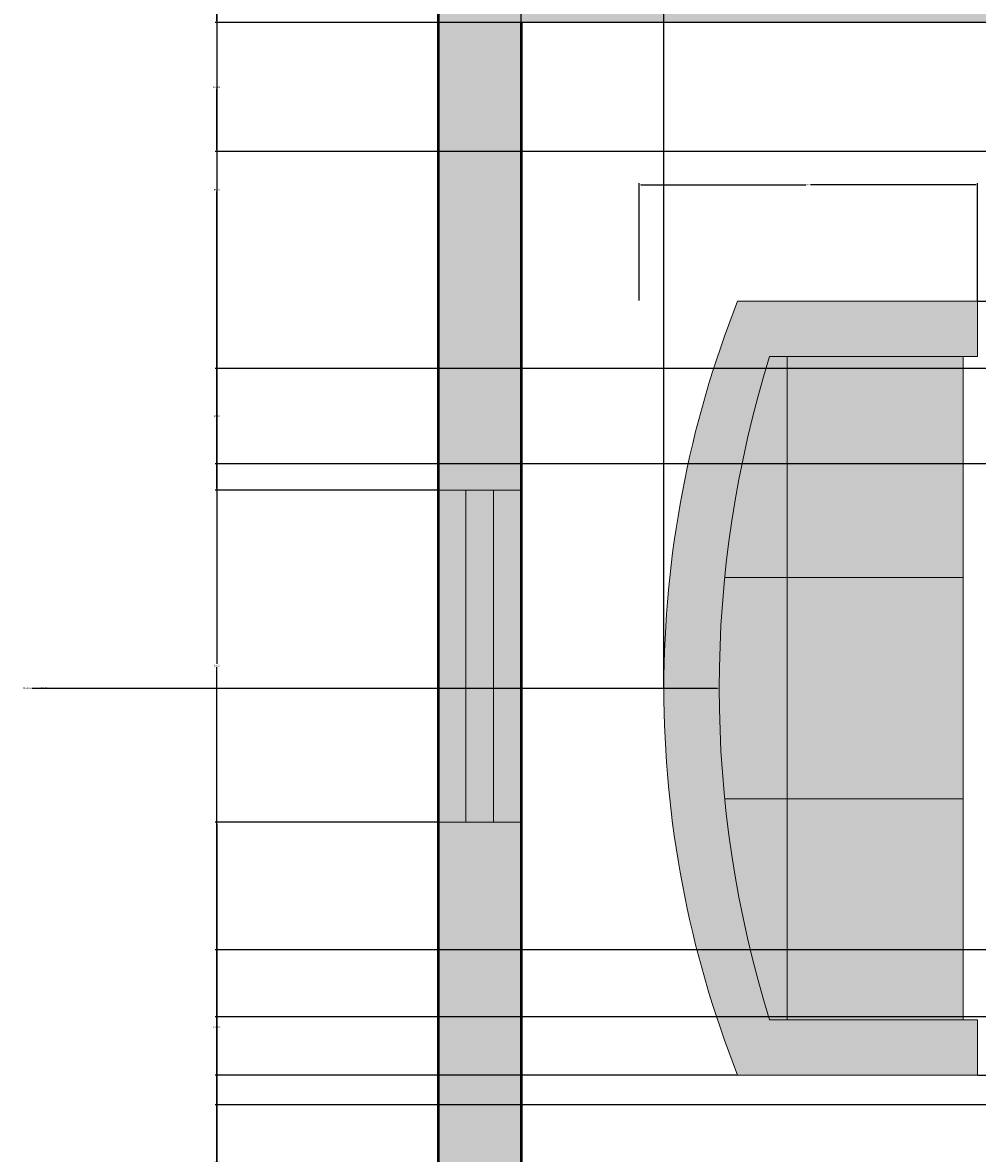
# Model space of a CAD drawing. Units: inches. Extents: x 1201 to 1754, y 247 to 775.
# Tile 2 of 10: x 1201 to 1305, y 435 to 557. Entities that reach past the tile are written whole.
import ezdxf

# ---------------------------------------------------------------- set-up
doc = ezdxf.new("R2010")
doc.units = ezdxf.units.IN
for name, color, linetype, lineweight in [('A-ANNO-DIMS', 2, 'Continuous', 18), ('A-FURN', 8, 'Continuous', 18), ('A-FURN-PATT', 9, 'Continuous', 13), ('A-GLAZ', 4, 'Continuous', 18), ('A-GLAZ-PATT', 9, 'Continuous', 13), ('A-WALL', 7, 'Continuous', 50), ('A-WALL-PATT', 9, 'Continuous', 13)]:
    doc.layers.add(name, color=color, linetype=linetype, lineweight=lineweight)
doc.styles.get("Standard").update_dxf_attribs({"font": 'arial.ttf'})
doc.dimstyles.get("Standard").update_dxf_attribs({"dimtxt": 0.18, "dimasz": 0.18, "dimexe": 0.18, "dimexo": 0.0625, "dimgap": 0.09, "dimtad": 0, "dimtih": 1, "dimtoh": 1, "dimdec": 4, "dimzin": 0, "dimdsep": 46, "dimtxsty": 'Standard', "dimcen": 0.09, "dimadec": 0, "dimazin": 0, "dimtfac": 1, "dimtdec": 4, "dimtofl": 0, "dimtmove": 0, "dimatfit": 3, "dimfxl": 1, "dimtolj": 1, "dimtzin": 0, "dimarcsym": 0})

# ---------------------------------------------------------------- blocks, each defined once
blk = doc.blocks.new('Sofa - Roundback 7 ft.')
for p, q in [((-12.00002, -32.4421), (-12.00003, -6.5971)), ((11.99997, -32.4421), (11.99998, -6.5971)), ((-36.000027, -34), (-36.000027, -11.4696)), ((35.99998, -34), (35.99998, -11.4696)), ((-35.999844, -13.3819), (35.9998, -13.3819)), ((-36.000027, -32.4421), (35.99998, -32.4421))]:
    blk.add_line(p, q)
for points in [[(-36.000027, -34), (-42.000027, -34), (-42.000027, -8)], [(41.99998, -8), (41.99998, -34), (35.99998, -34)]]:
    blk.add_lwpolyline(points)
for centre, radius, start, end in [((0, -114.25), 114.25, 68.43141, 111.5686), ((-0.00001, -127.1968), 121.1968, 72.72033, 107.2797)]:
    blk.add_arc(centre, radius, start, end)
blk = doc.blocks.new('WIN-36IN-PLAN')
for p, q in [((9, 36), (0, 36)), ((3, 0), (3, 36)), ((6, 0), (6, 36))]:
    blk.add_line(p, q)
blk.add_lwpolyline([(0, 36), (0, 0), (9, 0), (9, 36)])
blk = doc.blocks.new('*D37')
at = {"layer": 'A-ANNO-DIMS', "color": 0, "lineweight": -2, "transparency": 16777216}
for p, q in [((1305.08, 527.23), (1317.8, 527.23)), ((1317.62, 527.05), (1317.62, 485.41)), ((1317.62, 443.41), (1317.62, 485.04)), ((1305.08, 443.23), (1317.8, 443.23))]:
    blk.add_line(p, q, dxfattribs=at)
at = {"layer": 'A-ANNO-DIMS', "color": 0, "transparency": 16777216}
for points in [[(1317.59, 527.05), (1317.65, 527.05), (1317.62, 527.23)], [(1317.59, 443.41), (1317.65, 443.41), (1317.62, 443.23)]]:
    blk.add_solid(points, dxfattribs=at)
at = {"layer": 'Defpoints', "color": 0, "transparency": 16777216}
for p in [(1305.02, 527.23), (1317.62, 527.23), (1305.02, 443.23)]:
    blk.add_point(p, dxfattribs=at)
at = {"layer": 'A-ANNO-DIMS', "color": 0, "transparency": 16777216, "insert": (1317.62, 485.23), "char_height": 0.18, "attachment_point": 5}
blk.add_mtext('\\A1;SOFA 84', dxfattribs=at)
blk = doc.blocks.new('*D38')
at = {"layer": 'A-ANNO-DIMS', "color": 0, "lineweight": -2, "transparency": 16777216}
for p, q in [((1268.35, 527.29), (1268.35, 540.01)), ((1305.02, 527.29), (1305.02, 540.01)), ((1268.53, 539.83), (1286.46, 539.83)), ((1304.84, 539.83), (1286.9, 539.83))]:
    blk.add_line(p, q, dxfattribs=at)
at = {"layer": 'A-ANNO-DIMS', "color": 0, "transparency": 16777216}
for points in [[(1268.53, 539.86), (1268.53, 539.8), (1268.35, 539.83)], [(1304.84, 539.86), (1304.84, 539.8), (1305.02, 539.83)]]:
    blk.add_solid(points, dxfattribs=at)
at = {"layer": 'Defpoints', "color": 0, "transparency": 16777216}
for p in [(1268.35, 539.83), (1268.35, 527.23), (1305.02, 527.23)]:
    blk.add_point(p, dxfattribs=at)
at = {"layer": 'A-ANNO-DIMS', "color": 0, "transparency": 16777216, "insert": (1286.68, 539.83), "char_height": 0.18, "attachment_point": 5}
blk.add_mtext('\\A1;37', dxfattribs=at)
blk = doc.blocks.new('*D50')
at = {"layer": 'A-ANNO-DIMS', "color": 0, "lineweight": -2, "transparency": 16777216}
for p, q in [((1255.46, 557.44), (1222.33, 557.44)), ((1222.51, 557.26), (1222.51, 487.87)), ((1222.51, 418.12), (1222.51, 487.51)), ((1255.46, 417.94), (1222.33, 417.94))]:
    blk.add_line(p, q, dxfattribs=at)
at = {"layer": 'A-ANNO-DIMS', "color": 0, "transparency": 16777216}
for points in [[(1222.48, 557.26), (1222.54, 557.26), (1222.51, 557.44)], [(1222.48, 418.12), (1222.54, 418.12), (1222.51, 417.94)]]:
    blk.add_solid(points, dxfattribs=at)
at = {"layer": 'Defpoints', "color": 0, "transparency": 16777216}
for p in [(1255.52, 557.44), (1222.51, 417.94), (1255.52, 417.94)]:
    blk.add_point(p, dxfattribs=at)
at = {"layer": 'A-ANNO-DIMS', "color": 0, "transparency": 16777216, "insert": (1222.51, 487.69), "char_height": 0.18, "attachment_point": 5}
blk.add_mtext('\\A1;139.5', dxfattribs=at)
blk = doc.blocks.new('*D59')
at = {"layer": 'A-ANNO-DIMS', "color": 0, "lineweight": -2, "transparency": 16777216}
for p, q in [((1255.52, 418), (1255.52, 775.14)), ((1255.7, 774.96), (1330.24, 774.96)), ((1405.34, 774.96), (1330.8, 774.96)), ((1405.52, 418), (1405.52, 775.14))]:
    blk.add_line(p, q, dxfattribs=at)
at = {"layer": 'A-ANNO-DIMS', "color": 0, "transparency": 16777216}
for points in [[(1255.7, 774.99), (1255.7, 774.93), (1255.52, 774.96)], [(1405.34, 774.99), (1405.34, 774.93), (1405.52, 774.96)]]:
    blk.add_solid(points, dxfattribs=at)
at = {"layer": 'Defpoints', "color": 0, "transparency": 16777216}
for p in [(1405.52, 774.96), (1255.52, 417.94), (1405.52, 417.94)]:
    blk.add_point(p, dxfattribs=at)
at = {"layer": 'A-ANNO-DIMS', "color": 0, "transparency": 16777216, "insert": (1330.52, 774.96), "char_height": 0.18, "attachment_point": 5}
blk.add_mtext('\\A1;150', dxfattribs=at)
blk = doc.blocks.new('*D70')
at = {"layer": 'A-ANNO-DIMS', "color": 0, "lineweight": -2, "transparency": 16777216}
for p, q in [((1246.46, 470.7), (1222.33, 470.7)), ((1222.51, 470.52), (1222.51, 409.4)), ((1222.51, 347.93), (1222.51, 409.04)), ((1246.46, 347.75), (1222.33, 347.75))]:
    blk.add_line(p, q, dxfattribs=at)
at = {"layer": 'A-ANNO-DIMS', "color": 0, "transparency": 16777216}
for points in [[(1222.48, 470.52), (1222.54, 470.52), (1222.51, 470.7)], [(1222.48, 347.93), (1222.54, 347.93), (1222.51, 347.75)]]:
    blk.add_solid(points, dxfattribs=at)
at = {"layer": 'Defpoints', "color": 0, "transparency": 16777216}
for p in [(1222.51, 470.7), (1246.52, 470.7), (1246.52, 347.75)]:
    blk.add_point(p, dxfattribs=at)
at = {"layer": 'A-ANNO-DIMS', "color": 0, "transparency": 16777216, "insert": (1222.51, 409.22), "char_height": 0.18, "attachment_point": 5}
blk.add_mtext('\\A1;122.95', dxfattribs=at)
blk = doc.blocks.new('*D71')
at = {"layer": 'A-ANNO-DIMS', "color": 0, "lineweight": -2, "transparency": 16777216}
for p, q in [((1246.46, 571.89), (1222.33, 571.89)), ((1222.51, 571.71), (1222.51, 539.47)), ((1222.51, 506.88), (1222.51, 539.11)), ((1246.46, 506.7), (1222.33, 506.7))]:
    blk.add_line(p, q, dxfattribs=at)
at = {"layer": 'A-ANNO-DIMS', "color": 0, "transparency": 16777216}
for points in [[(1222.48, 571.71), (1222.54, 571.71), (1222.51, 571.89)], [(1222.48, 506.88), (1222.54, 506.88), (1222.51, 506.7)]]:
    blk.add_solid(points, dxfattribs=at)
at = {"layer": 'Defpoints', "color": 0, "transparency": 16777216}
for p in [(1222.51, 571.89), (1246.52, 571.89), (1246.52, 506.7)]:
    blk.add_point(p, dxfattribs=at)
at = {"layer": 'A-ANNO-DIMS', "color": 0, "transparency": 16777216, "insert": (1222.51, 539.29), "char_height": 0.18, "attachment_point": 5}
blk.add_mtext('\\A1;65.19', dxfattribs=at)
blk = doc.blocks.new('*D75')
at = {"layer": 'A-ANNO-DIMS', "color": 0, "lineweight": -2, "transparency": 16777216}
for p, q in [((1717.46, 557.44), (1222.33, 557.44)), ((1222.51, 557.26), (1222.51, 550.62)), ((1222.51, 543.62), (1222.51, 550.26)), ((1717.46, 543.44), (1222.33, 543.44))]:
    blk.add_line(p, q, dxfattribs=at)
at = {"layer": 'A-ANNO-DIMS', "color": 0, "transparency": 16777216}
for points in [[(1222.48, 557.26), (1222.54, 557.26), (1222.51, 557.44)], [(1222.48, 543.62), (1222.54, 543.62), (1222.51, 543.44)]]:
    blk.add_solid(points, dxfattribs=at)
at = {"layer": 'Defpoints', "color": 0, "transparency": 16777216}
for p in [(1222.51, 557.44), (1717.52, 557.44), (1717.52, 543.44)]:
    blk.add_point(p, dxfattribs=at)
at = {"layer": 'A-ANNO-DIMS', "color": 0, "transparency": 16777216, "insert": (1222.51, 550.44), "char_height": 0.18, "attachment_point": 5}
blk.add_mtext('\\A1;14.005', dxfattribs=at)
blk = doc.blocks.new('*D83')
at = {"layer": 'A-ANNO-DIMS', "color": 0, "lineweight": -2, "transparency": 16777216}
for p, q in [((1471.46, 561.97), (1222.33, 561.97)), ((1222.51, 561.79), (1222.51, 559.89)), ((1222.51, 557.62), (1222.51, 559.52)), ((1471.46, 557.44), (1222.33, 557.44))]:
    blk.add_line(p, q, dxfattribs=at)
at = {"layer": 'A-ANNO-DIMS', "color": 0, "transparency": 16777216}
for points in [[(1222.48, 561.79), (1222.54, 561.79), (1222.51, 561.97)], [(1222.48, 557.62), (1222.54, 557.62), (1222.51, 557.44)]]:
    blk.add_solid(points, dxfattribs=at)
at = {"layer": 'Defpoints', "color": 0, "transparency": 16777216}
for p in [(1222.51, 561.97), (1471.52, 561.97), (1471.52, 557.44)]:
    blk.add_point(p, dxfattribs=at)
at = {"layer": 'A-ANNO-DIMS', "color": 0, "transparency": 16777216, "insert": (1222.51, 559.71), "char_height": 0.18, "attachment_point": 5}
blk.add_mtext('\\A1;4.528', dxfattribs=at)
blk = doc.blocks.new('*D93')
at = {"layer": 'A-ANNO-DIMS', "color": 0, "lineweight": -2, "transparency": 16777216}
for p, q in [((1278.95, 443.23), (1222.33, 443.23)), ((1222.51, 443.05), (1222.51, 430.77)), ((1222.51, 418.12), (1222.51, 430.4)), ((1255.46, 417.94), (1222.33, 417.94))]:
    blk.add_line(p, q, dxfattribs=at)
at = {"layer": 'A-ANNO-DIMS', "color": 0, "transparency": 16777216}
for points in [[(1222.48, 443.05), (1222.54, 443.05), (1222.51, 443.23)], [(1222.48, 418.12), (1222.54, 418.12), (1222.51, 417.94)]]:
    blk.add_solid(points, dxfattribs=at)
at = {"layer": 'Defpoints', "color": 0, "transparency": 16777216}
for p in [(1222.51, 443.23), (1279.02, 443.23), (1255.52, 417.94)]:
    blk.add_point(p, dxfattribs=at)
at = {"layer": 'A-ANNO-DIMS', "color": 0, "transparency": 16777216, "insert": (1222.51, 430.58), "char_height": 0.18, "attachment_point": 5}
blk.add_mtext('\\A1;25.285', dxfattribs=at)
blk = doc.blocks.new('*D95')
at = {"layer": 'A-ANNO-DIMS', "color": 0, "lineweight": -2, "transparency": 16777216}
for p, q in [((1366.15, 449.58), (1222.33, 449.58)), ((1222.51, 449.4), (1222.51, 433.94)), ((1222.51, 418.12), (1222.51, 433.58)), ((1405.46, 417.94), (1222.33, 417.94))]:
    blk.add_line(p, q, dxfattribs=at)
at = {"layer": 'A-ANNO-DIMS', "color": 0, "transparency": 16777216}
for points in [[(1222.48, 449.4), (1222.54, 449.4), (1222.51, 449.58)], [(1222.48, 418.12), (1222.54, 418.12), (1222.51, 417.94)]]:
    blk.add_solid(points, dxfattribs=at)
at = {"layer": 'Defpoints', "color": 0, "transparency": 16777216}
for p in [(1366.21, 449.58), (1222.51, 417.94), (1405.52, 417.94)]:
    blk.add_point(p, dxfattribs=at)
at = {"layer": 'A-ANNO-DIMS', "color": 0, "transparency": 16777216, "insert": (1222.51, 433.76), "char_height": 0.18, "attachment_point": 5}
blk.add_mtext('\\A1;31.64', dxfattribs=at)
blk = doc.blocks.new('*D96')
at = {"layer": 'A-ANNO-DIMS', "color": 0, "lineweight": -2, "transparency": 16777216}
for p, q in [((1714.98, 456.83), (1222.33, 456.83)), ((1222.51, 456.65), (1222.51, 448.61)), ((1222.51, 440.21), (1222.51, 448.25)), ((1717.46, 440.03), (1222.33, 440.03))]:
    blk.add_line(p, q, dxfattribs=at)
at = {"layer": 'A-ANNO-DIMS', "color": 0, "transparency": 16777216}
for points in [[(1222.48, 456.65), (1222.54, 456.65), (1222.51, 456.83)], [(1222.48, 440.21), (1222.54, 440.21), (1222.51, 440.03)]]:
    blk.add_solid(points, dxfattribs=at)
at = {"layer": 'Defpoints', "color": 0, "transparency": 16777216}
for p in [(1222.51, 456.83), (1715.05, 456.83), (1717.52, 440.03)]:
    blk.add_point(p, dxfattribs=at)
at = {"layer": 'A-ANNO-DIMS', "color": 0, "transparency": 16777216, "insert": (1222.51, 448.43), "char_height": 0.18, "attachment_point": 5}
blk.add_mtext('\\A1;16.793', dxfattribs=at)
blk = doc.blocks.new('*D97')
at = {"layer": 'A-ANNO-DIMS', "color": 0, "lineweight": -2, "transparency": 16777216}
for p, q in [((1255.52, 506.76), (1255.52, 775.14)), ((1255.7, 774.96), (1262.81, 774.96)), ((1270.84, 774.96), (1263.72, 774.96)), ((1271.02, 485.29), (1271.02, 775.14))]:
    blk.add_line(p, q, dxfattribs=at)
at = {"layer": 'A-ANNO-DIMS', "color": 0, "transparency": 16777216}
for points in [[(1255.7, 774.99), (1255.7, 774.93), (1255.52, 774.96)], [(1270.84, 774.99), (1270.84, 774.93), (1271.02, 774.96)]]:
    blk.add_solid(points, dxfattribs=at)
at = {"layer": 'Defpoints', "color": 0, "transparency": 16777216}
for p in [(1271.02, 774.96), (1255.52, 506.7), (1271.02, 485.23)]:
    blk.add_point(p, dxfattribs=at)
at = {"layer": 'A-ANNO-DIMS', "color": 0, "transparency": 16777216, "insert": (1263.27, 774.96), "char_height": 0.18, "attachment_point": 5}
blk.add_mtext('\\A1;15.496', dxfattribs=at)
blk = doc.blocks.new('*D99')
at = {"layer": 'A-ANNO-DIMS', "color": 0, "lineweight": -2, "transparency": 16777216}
for p, q in [((1379.64, 519.9), (1222.33, 519.9)), ((1222.51, 519.72), (1222.51, 514.93)), ((1222.51, 509.76), (1222.51, 514.56)), ((1366.15, 509.58), (1222.33, 509.58))]:
    blk.add_line(p, q, dxfattribs=at)
at = {"layer": 'A-ANNO-DIMS', "color": 0, "transparency": 16777216}
for points in [[(1222.48, 519.72), (1222.54, 519.72), (1222.51, 519.9)], [(1222.48, 509.76), (1222.54, 509.76), (1222.51, 509.58)]]:
    blk.add_solid(points, dxfattribs=at)
at = {"layer": 'Defpoints', "color": 0, "transparency": 16777216}
for p in [(1222.51, 519.9), (1379.71, 519.9), (1366.21, 509.58)]:
    blk.add_point(p, dxfattribs=at)
at = {"layer": 'A-ANNO-DIMS', "color": 0, "transparency": 16777216, "insert": (1222.51, 514.74), "char_height": 0.18, "attachment_point": 5}
blk.add_mtext('\\A1;10.32', dxfattribs=at)
blk = doc.blocks.new('*D100')
at = {"layer": 'A-ANNO-DIMS', "color": 0, "lineweight": -2, "transparency": 16777216}
for p, q in [((1204.3, 485.23), (1276.84, 485.23)), ((1398.12, 485.23), (1398.3, 485.23)), ((1398.21, 485.14), (1398.21, 485.32))]:
    blk.add_line(p, q, dxfattribs=at)
at = {"layer": 'A-ANNO-DIMS', "color": 0, "transparency": 16777216}
blk.add_solid([(1276.84, 485.26), (1276.84, 485.2), (1277.02, 485.23)], dxfattribs=at)
at = {"layer": 'Defpoints', "color": 0, "transparency": 16777216}
for p in [(1277.02, 485.23), (1398.21, 485.23)]:
    blk.add_point(p, dxfattribs=at)
at = {"layer": 'A-ANNO-DIMS', "color": 0, "transparency": 16777216, "insert": (1203.82, 485.23), "char_height": 0.18, "attachment_point": 5}
blk.add_mtext('\\A1;R121.2', dxfattribs=at)
blk = doc.blocks.new('*D101')
at = {"layer": 'A-ANNO-DIMS', "color": 0, "lineweight": -2, "transparency": 16777216}
for p, q in [((1202.47, 485.23), (1270.84, 485.23)), ((1385.18, 485.23), (1385.36, 485.23)), ((1385.27, 485.14), (1385.27, 485.32))]:
    blk.add_line(p, q, dxfattribs=at)
at = {"layer": 'A-ANNO-DIMS', "color": 0, "transparency": 16777216}
blk.add_solid([(1270.84, 485.26), (1270.84, 485.2), (1271.02, 485.23)], dxfattribs=at)
at = {"layer": 'Defpoints', "color": 0, "transparency": 16777216}
for p in [(1271.02, 485.23), (1385.27, 485.23)]:
    blk.add_point(p, dxfattribs=at)
at = {"layer": 'A-ANNO-DIMS', "color": 0, "transparency": 16777216, "insert": (1201.92, 485.23), "char_height": 0.18, "attachment_point": 5}
blk.add_mtext('\\A1;R114.25', dxfattribs=at)

msp = doc.modelspace()

# ---------------------------------------------------------------- hatches: boundary and pattern name
at = {"layer": 'A-FURN-PATT'}
h = msp.add_hatch(color=256, dxfattribs=at)
h.dxf.hatch_style = 1
h.paths.add_polyline_path([(1373.7057, 540.5217), (1349.7056, 540.5217), (1349.7056, 521.4615), (1373.7057, 521.4615)], flags=17)
h.paths.add_polyline_path([(1349.7056, 540.5217), (1325.7056, 540.5217), (1325.7056, 521.4615), (1349.7056, 521.4615)], flags=17)
h.paths.add_polyline_path([(1349.7056, 547.9035, 0.11251869), (1325.7056, 542.4334), (1325.7056, 540.5217), (1349.7056, 540.5217)], flags=17)
h.paths.add_polyline_path([(1349.7056, 547.9035), (1349.7056, 540.5217), (1373.7057, 540.5217), (1373.7057, 542.4333, 0.11251889)], flags=17)
h.paths.add_polyline_path([(1319.7056, 545.9034), (1319.7056, 519.9035), (1325.7056, 519.9035), (1325.7056, 542.4334, -0.22792319), (1373.7057, 542.4333), (1373.7057, 540.5217), (1373.7057, 521.4615), (1373.7057, 519.9035), (1379.7057, 519.9035), (1379.7057, 545.9034, 0.26666697)])
h.paths.add_polyline_path([(1303.4586, 521.2267), (1284.3984, 521.2267), (1284.3984, 497.2267), (1303.4586, 497.2267)], flags=17)
h.paths.add_polyline_path([(1303.4586, 497.2267), (1284.3984, 497.2267), (1284.3984, 473.2267), (1303.4586, 473.2267)], flags=17)
h.paths.add_polyline_path([(1303.4586, 473.2267), (1284.3984, 473.2267), (1284.3984, 449.2267), (1303.4586, 449.2267)], flags=17)
h.paths.add_polyline_path([(1282.4866, 521.2267), (1305.0165, 521.2267), (1305.0165, 527.2267), (1279.0165, 527.2267, 0.19047621), (1279.0165, 443.2267), (1305.0165, 443.2267), (1305.0165, 449.2267), (1282.4866, 449.2267, -0.15194781)])
h.paths.add_polyline_path([(1284.3984, 497.2267), (1277.612, 497.2267, 0.04962821), (1277.612, 473.2267), (1284.3984, 473.2267)], flags=17)
h.paths.add_polyline_path([(1284.3984, 521.2267), (1282.4866, 521.2267, 0.05064665), (1277.612, 497.2267), (1284.3984, 497.2267)], flags=17)
h.paths.add_polyline_path([(1284.3984, 473.2267), (1277.612, 473.2267, 0.05064665), (1282.4866, 449.2267), (1284.3984, 449.2267)], flags=17)
at = {"layer": 'A-GLAZ-PATT'}
h = msp.add_hatch(color=256, dxfattribs=at)
h.dxf.hatch_style = 1
h.set_gradient(color1=(0, 0, 255), color2=(255, 255, 0), name='CURVED')
h.paths.add_polyline_path([(1255.5208, 506.6967), (1252.5208, 506.6967), (1252.5208, 470.6967), (1255.5208, 470.6967)])
h.paths.add_polyline_path([(1252.5208, 506.6967), (1249.5208, 506.6967), (1249.5208, 470.6967), (1252.5208, 470.6967)])
h.paths.add_polyline_path([(1249.5208, 506.6967), (1246.5208, 506.6967), (1246.5208, 470.6967), (1249.5208, 470.6967)])
at = {"layer": 'A-WALL-PATT'}
h = msp.add_hatch(color=256, dxfattribs=at)
h.dxf.hatch_style = 1
h.paths.add_polyline_path([(1255.5208, 741.9415), (1471.5208, 741.9415), (1471.5208, 684.2327), (1471.5208, 602.9415), (1477.5208, 602.9415), (1477.5208, 669.9415), (1618.5208, 669.9415), (1618.5208, 674.4415), (1477.5208, 674.4415), (1477.5208, 741.9415), (1481.2969, 741.9415), (1481.2969, 750.9415), (1246.5208, 750.9415), (1246.5208, 700.7954), (1255.5208, 700.7954)])
h.paths.add_polyline_path([(1255.5208, 557.4415), (1399.5208, 557.4415), (1399.5208, 617.4415), (1423.5208, 617.4415), (1423.5208, 621.9415), (1392.0208, 621.9415), (1392.0208, 617.4415), (1395.0208, 617.4415), (1395.0208, 561.9415), (1255.5208, 561.9415), (1255.5208, 571.8878), (1246.5208, 571.8878), (1246.5208, 506.6967), (1255.5208, 506.6967)])
h.paths.add_polyline_path([(1255.5208, 664.7954), (1246.5208, 664.7954), (1246.5208, 595.8878), (1255.398, 595.8878), (1255.398, 617.4415), (1315.398, 617.4415), (1356.0208, 617.4415), (1356.0208, 618.0127), (1356.0208, 621.9415), (1255.5208, 621.9415), (1255.5208, 629.6628)])
h.paths.add_polyline_path([(1255.5208, 470.6967), (1246.5208, 470.6967), (1246.5208, 347.7487), (1255.5208, 347.7487), (1255.5208, 413.4415), (1405.5208, 413.4415), (1405.5208, 417.9415), (1255.5208, 417.9415)])
h.paths.add_polyline_path([(1290.9481, 279.9415), (1255.5208, 279.9415), (1255.5208, 311.7487), (1246.5208, 311.7487), (1246.5208, 270.9415), (1290.9481, 270.9415)])
h.paths.add_polyline_path([(1486.5907, 279.9415), (1477.5208, 279.9415), (1477.5208, 417.9415), (1468.5208, 417.9415), (1468.5208, 413.4415), (1471.5208, 413.4415), (1471.5208, 279.9415), (1399.0105, 279.9415), (1399.0105, 270.9415), (1486.5907, 270.9415)])
h.paths.add_polyline_path([(1563.0208, 279.9415), (1542.0208, 279.9415), (1542.0208, 417.9415), (1501.5208, 417.9415), (1501.5208, 413.4415), (1513.81, 413.4415), (1513.8125, 413.6987), (1537.8114, 413.4623), (1537.5208, 383.9637), (1537.5208, 279.9415), (1522.5907, 279.9415), (1522.5907, 270.9415), (1563.0208, 270.9415)])
h.paths.add_polyline_path([(1726.5208, 404.0342), (1717.5208, 404.0342), (1717.5208, 279.9415), (1641.0208, 279.9415), (1641.0208, 270.9415), (1726.5208, 270.9415)])
h.paths.add_polyline_path([(1726.5208, 507.4363), (1717.5208, 507.4363), (1717.5208, 440.0342), (1726.5208, 440.0342)])
h.paths.add_polyline_path([(1726.5208, 611.6009), (1717.5208, 611.6009), (1717.5208, 561.9415), (1477.5208, 561.9415), (1471.5208, 561.9692), (1471.5208, 557.4415), (1717.5208, 557.4415), (1717.5208, 543.4363), (1726.5208, 543.4363)])
h.paths.add_polyline_path([(1726.5208, 750.9415), (1505.2969, 750.9415), (1505.2969, 741.9415), (1697.6884, 741.9415), (1697.6884, 741.9922), (1718.6884, 741.9922), (1718.6884, 733.9922), (1717.5208, 733.9922), (1717.5208, 674.4415), (1660.5208, 674.4415), (1660.5208, 669.9415), (1717.5208, 669.9415), (1717.5208, 647.6009), (1726.5208, 647.6009)])

# ---------------------------------------------------------------- linework, layer by layer
at = {"layer": 'A-WALL'}
msp.add_line((1255.5208, 557.4415), (1255.5208, 417.9415), dxfattribs=at)
msp.add_lwpolyline([(1638.0208, 270.9415), (1726.5208, 270.9415), (1726.5208, 750.9415), (1246.5208, 750.9415), (1246.5208, 270.9415), (1566.0208, 270.9415)], dxfattribs=at)

# ---------------------------------------------------------------- block references
at = {"layer": 'A-FURN', "rotation": 90}
msp.add_blockref('Sofa - Roundback 7 ft.', (1271.0165, 485.2267), dxfattribs=at)
at = {"layer": 'A-GLAZ'}
msp.add_blockref('WIN-36IN-PLAN', (1246.5208, 470.6967), dxfattribs=at)

# ---------------------------------------------------------------- dimensions: what is measured, and where the dimension line sits
at = {"layer": 'A-ANNO-DIMS'}
for base, p1, p2, override, picture, middle in [((1405.5208, 774.9565), (1255.5208, 417.9415), (1405.5208, 417.9415), {"dimdec": 0, "dimlfac": 1, "dimrnd": 0, "dimzin": 0, "dimdsep": 46, "dimlunit": 2}, '*D59', (1330.5208, 774.9565)), ((1271.0165, 774.9565), (1255.5208, 506.6967), (1271.0165, 485.2267), {"dimdec": 3, "dimlfac": 1, "dimrnd": 0, "dimzin": 0, "dimdsep": 46, "dimlunit": 2}, '*D97', (1263.2686, 774.9565))]:
    dim = msp.add_linear_dim(base=base, p1=p1, p2=p2, dimstyle='Standard', override=override, dxfattribs=at)
    dim.commit()
    dim.dimension.update_dxf_attribs({"geometry": picture, "text_midpoint": middle})
for base, p1, p2, angle, override, picture, middle in [((1222.5058, 571.8878), (1246.5208, 506.6967), (1246.5208, 571.8878), 90, {"dimdec": 2, "dimlfac": 1, "dimrnd": 0, "dimzin": 0, "dimdsep": 46, "dimlunit": 2}, '*D71', (1222.5058, 539.2922)), ((1222.5058, 561.9692), (1471.5208, 557.4415), (1471.5208, 561.9692), 90, {"dimdec": 3, "dimlfac": 1, "dimrnd": 0, "dimzin": 0, "dimdsep": 46, "dimlunit": 2}, '*D83', (1222.5058, 559.7053)), ((1222.5058, 557.4415), (1717.5208, 543.4363), (1717.5208, 557.4415), 90, {"dimdec": 3, "dimlfac": 1, "dimrnd": 0, "dimzin": 0, "dimdsep": 46, "dimlunit": 2}, '*D75', (1222.5058, 550.4389)), ((1222.5058, 417.9415), (1255.5208, 557.4415), (1255.5208, 417.9415), 90, {"dimdec": 1, "dimlfac": 1, "dimrnd": 0, "dimzin": 0, "dimdsep": 46, "dimlunit": 2}, '*D50', (1222.5058, 487.6915)), ((1268.3498, 539.8267), (1305.0165, 527.2267), (1268.3498, 527.2267), 180, {"dimdec": 0, "dimlfac": 1, "dimrnd": 0, "dimzin": 0, "dimdsep": 46, "dimlunit": 2}, '*D38', (1286.6832, 539.8267)), ((1222.5058, 519.9035), (1366.2113, 509.5839), (1379.7057, 519.9035), 90, {"dimdec": 2, "dimlfac": 1, "dimrnd": 0, "dimzin": 0, "dimdsep": 46, "dimlunit": 2}, '*D99', (1222.5058, 514.7437)), ((1222.5058, 470.6967), (1246.5208, 347.7487), (1246.5208, 470.6967), 90, {"dimdec": 2, "dimlfac": 1, "dimrnd": 0, "dimzin": 0, "dimdsep": 46, "dimlunit": 2}, '*D70', (1222.5058, 409.2227)), ((1222.5058, 456.8273), (1717.5208, 440.0342), (1715.0469, 456.8273), 90, {"dimdec": 3, "dimlfac": 1, "dimrnd": 0, "dimzin": 0, "dimdsep": 46, "dimlunit": 2}, '*D96', (1222.5058, 448.4308)), ((1222.5058, 417.9415), (1366.2113, 449.5839), (1405.5208, 417.9415), 90, {"dimdec": 2, "dimlfac": 1, "dimrnd": 0, "dimzin": 0, "dimdsep": 46, "dimlunit": 2}, '*D95', (1222.5058, 433.7627)), ((1222.5058, 443.2267), (1255.5208, 417.9415), (1279.0165, 443.2267), 90, {"dimdec": 3, "dimlfac": 1, "dimrnd": 0, "dimzin": 0, "dimdsep": 46, "dimlunit": 2}, '*D93', (1222.5058, 430.5841))]:
    dim = msp.add_linear_dim(base=base, p1=p1, p2=p2, angle=angle, dimstyle='Standard', override=override, dxfattribs=at)
    dim.commit()
    dim.dimension.update_dxf_attribs({"geometry": picture, "text_midpoint": middle})
dim = msp.add_linear_dim(base=(1317.6165, 527.2267), p1=(1305.0165, 443.2267), p2=(1305.0165, 527.2267), angle=90, text='SOFA <>', dimstyle='Standard', override={"dimdec": 0, "dimlfac": 1, "dimrnd": 0, "dimzin": 0, "dimdsep": 46, "dimlunit": 2}, dxfattribs=at)
dim.commit()
dim.dimension.update_dxf_attribs({"geometry": '*D37', "text_midpoint": (1317.6165, 485.2267)})
for center, mpoint, override, picture, middle in [((1385.2665, 485.2267), (1271.0165, 485.227), {"dimdec": 2, "dimlfac": 1, "dimrnd": 0, "dimzin": 0, "dimdsep": 46, "dimlunit": 2}, '*D101', (1202.4665, 485.2272)), ((1398.2133, 485.2267), (1277.0165, 485.227), {"dimdec": 1, "dimlfac": 1, "dimrnd": 0, "dimzin": 0, "dimdsep": 46, "dimlunit": 2}, '*D100', (1204.2984, 485.2272))]:
    dim = msp.add_radius_dim(center=center, mpoint=mpoint, dimstyle='Standard', override=override, dxfattribs=at)
    dim.commit()
    dim.dimension.update_dxf_attribs({"geometry": picture, "text_midpoint": middle, "dimtype": 164})

doc.saveas('drawing.dxf')
